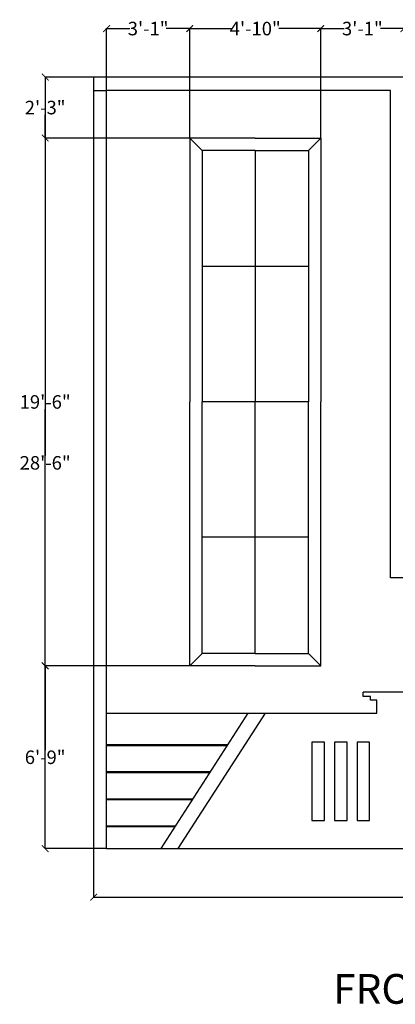
# Model space of a CAD drawing. Units: inches. Extents: x 2278 to 7495, y -71 to 1198.
# Tile 8 of 44: x 4704 to 4871, y -71 to 366. Entities that reach past the tile are written whole.
import ezdxf

# ---------------------------------------------------------------- set-up
doc = ezdxf.new("R2010")
doc.units = ezdxf.units.IN
doc.header["$MEASUREMENT"] = 0
for name, color, linetype, lineweight in [('A-ANNO-DIMS', 2, 'Continuous', 18), ('A-ANNO-TEXT', 7, 'Continuous', 25), ('A-ELEV', 7, 'Continuous', 25)]:
    doc.layers.add(name, color=color, linetype=linetype, lineweight=lineweight)
doc.styles.get("Standard").update_dxf_attribs({"font": 'arial.ttf'})
doc.dimstyles.get("Standard").update_dxf_attribs({"dimtxt": 6, "dimasz": 3, "dimexe": 0.18, "dimexo": 0.0625, "dimgap": 0.09, "dimtad": 0, "dimtih": 1, "dimtoh": 1, "dimdec": 0, "dimzin": 0, "dimdsep": 46, "dimlunit": 3, "dimtxsty": 'Standard', "dimblk": 'ARCHTICK', "dimcen": 0.09, "dimadec": 0, "dimazin": 0, "dimtfac": 1, "dimtdec": 0, "dimtofl": 0, "dimtmove": 0, "dimatfit": 3, "dimfxl": 1, "dimtolj": 1, "dimtzin": 0, "dimarcsym": 0})

# ---------------------------------------------------------------- blocks, each defined once
blk = doc.blocks.new('_ArchTick')
at = {"color": 0, "linetype": 'ByBlock', "const_width": 0.15}
blk.add_lwpolyline([(-0.5, -0.5), (0.5, 0.5)], dxfattribs=at)
blk = doc.blocks.new('*D123')
at = {"layer": 'A-ANNO-DIMS', "color": 0, "lineweight": -2, "transparency": 16777216}
for p, q in [((4736.95, 340.16), (4736.95, -23.43)), ((5145.68, -1.81), (5145.68, -23.43)), ((4736.95, -23.25), (4923.93, -23.25)), ((5145.68, -23.25), (4958.7, -23.25))]:
    blk.add_line(p, q, dxfattribs=at)
at = {"layer": 'Defpoints', "color": 0, "transparency": 16777216}
for p in [(4736.95, 340.22), (5145.68, -1.75), (5145.68, -23.25)]:
    blk.add_point(p, dxfattribs=at)
at = {"layer": 'A-ANNO-DIMS', "color": 0, "lineweight": -2, "transparency": 16777216, "xscale": 3, "yscale": 3, "zscale": 3, "rotation": 180}
blk.add_blockref('_ArchTick', (4736.95, -23.25), dxfattribs=at)
at = {"layer": 'A-ANNO-DIMS', "color": 0, "lineweight": -2, "transparency": 16777216, "xscale": 3, "yscale": 3, "zscale": 3}
blk.add_blockref('_ArchTick', (5145.68, -23.25), dxfattribs=at)
at = {"layer": 'A-ANNO-DIMS', "color": 0, "transparency": 16777216, "insert": (4941.31, -23.25), "char_height": 6, "attachment_point": 5}
blk.add_mtext('\\A1;34\'-0 1/2"', dxfattribs=at)
blk = doc.blocks.new('*D124')
at = {"layer": 'A-ANNO-DIMS', "color": 0, "lineweight": -2, "transparency": 16777216}
for p, q in [((4742.68, 334.28), (4742.68, 361.9)), ((4742.68, 361.72), (4753.08, 361.72)), ((4779.62, 361.72), (4769.21, 361.72)), ((4779.62, 313.27), (4779.62, 361.9))]:
    blk.add_line(p, q, dxfattribs=at)
at = {"layer": 'Defpoints', "color": 0, "transparency": 16777216}
for p in [(4779.62, 361.72), (4742.68, 334.22), (4779.62, 313.21)]:
    blk.add_point(p, dxfattribs=at)
at = {"layer": 'A-ANNO-DIMS', "color": 0, "lineweight": -2, "transparency": 16777216, "xscale": 3, "yscale": 3, "zscale": 3, "rotation": 180}
blk.add_blockref('_ArchTick', (4742.68, 361.72), dxfattribs=at)
at = {"layer": 'A-ANNO-DIMS', "color": 0, "lineweight": -2, "transparency": 16777216, "xscale": 3, "yscale": 3, "zscale": 3}
blk.add_blockref('_ArchTick', (4779.62, 361.72), dxfattribs=at)
at = {"layer": 'A-ANNO-DIMS', "color": 0, "transparency": 16777216, "insert": (4761.15, 361.72), "char_height": 6, "attachment_point": 5}
blk.add_mtext('\\A1;3\'-1"', dxfattribs=at)
blk = doc.blocks.new('*D125')
at = {"layer": 'A-ANNO-DIMS', "color": 0, "lineweight": -2, "transparency": 16777216}
for p, q in [((4779.62, 313.27), (4779.62, 361.9)), ((4779.62, 361.72), (4798.16, 361.72)), ((4837.74, 361.72), (4819.19, 361.72)), ((4837.74, 313.27), (4837.74, 361.9))]:
    blk.add_line(p, q, dxfattribs=at)
at = {"layer": 'Defpoints', "color": 0, "transparency": 16777216}
for p in [(4837.74, 361.72), (4779.62, 313.21), (4837.74, 313.21)]:
    blk.add_point(p, dxfattribs=at)
at = {"layer": 'A-ANNO-DIMS', "color": 0, "lineweight": -2, "transparency": 16777216, "xscale": 3, "yscale": 3, "zscale": 3, "rotation": 180}
blk.add_blockref('_ArchTick', (4779.62, 361.72), dxfattribs=at)
at = {"layer": 'A-ANNO-DIMS', "color": 0, "lineweight": -2, "transparency": 16777216, "xscale": 3, "yscale": 3, "zscale": 3}
blk.add_blockref('_ArchTick', (4837.74, 361.72), dxfattribs=at)
at = {"layer": 'A-ANNO-DIMS', "color": 0, "transparency": 16777216, "insert": (4808.68, 361.72), "char_height": 6, "attachment_point": 5}
blk.add_mtext('\\A1;4\'-10"', dxfattribs=at)
blk = doc.blocks.new('*D126')
at = {"layer": 'A-ANNO-DIMS', "color": 0, "lineweight": -2, "transparency": 16777216}
for p, q in [((4837.74, 313.27), (4837.74, 361.9)), ((4837.74, 361.72), (4848.14, 361.72)), ((4874.68, 361.72), (4864.27, 361.72)), ((4874.68, 99.32), (4874.68, 361.9))]:
    blk.add_line(p, q, dxfattribs=at)
at = {"layer": 'Defpoints', "color": 0, "transparency": 16777216}
for p in [(4874.68, 361.72), (4837.74, 313.21), (4874.68, 99.25)]:
    blk.add_point(p, dxfattribs=at)
at = {"layer": 'A-ANNO-DIMS', "color": 0, "lineweight": -2, "transparency": 16777216, "xscale": 3, "yscale": 3, "zscale": 3, "rotation": 180}
blk.add_blockref('_ArchTick', (4837.74, 361.72), dxfattribs=at)
at = {"layer": 'A-ANNO-DIMS', "color": 0, "lineweight": -2, "transparency": 16777216, "xscale": 3, "yscale": 3, "zscale": 3}
blk.add_blockref('_ArchTick', (4874.68, 361.72), dxfattribs=at)
at = {"layer": 'A-ANNO-DIMS', "color": 0, "transparency": 16777216, "insert": (4856.21, 361.72), "char_height": 6, "attachment_point": 5}
blk.add_mtext('\\A1;3\'-1"', dxfattribs=at)
blk = doc.blocks.new('*D132')
at = {"layer": 'A-ANNO-DIMS', "color": 0, "lineweight": -2, "transparency": 16777216}
for p, q in [((4779.55, 79.26), (4715.27, 79.26)), ((4715.45, 79.26), (4715.45, 41.91)), ((4715.45, -1.75), (4715.45, 35.61)), ((4742.61, -1.75), (4715.27, -1.75))]:
    blk.add_line(p, q, dxfattribs=at)
at = {"layer": 'Defpoints', "color": 0, "transparency": 16777216}
for p in [(4715.45, 79.26), (4779.62, 79.26), (4742.68, -1.75)]:
    blk.add_point(p, dxfattribs=at)
at = {"layer": 'A-ANNO-DIMS', "color": 0, "lineweight": -2, "transparency": 16777216, "xscale": 3, "yscale": 3, "zscale": 3}
for p, rotation in [((4715.45, 79.26), 90), ((4715.45, -1.75), 270)]:
    blk.add_blockref('_ArchTick', p, dxfattribs=dict(at, rotation=rotation))
at = {"layer": 'A-ANNO-DIMS', "color": 0, "transparency": 16777216, "insert": (4715.45, 38.76), "char_height": 6, "attachment_point": 5}
blk.add_mtext('\\A1;6\'-9"', dxfattribs=at)
blk = doc.blocks.new('*D133')
at = {"layer": 'A-ANNO-DIMS', "color": 0, "lineweight": -2, "transparency": 16777216}
for p, q in [((4779.55, 313.21), (4715.27, 313.21)), ((4715.45, 313.21), (4715.45, 199.39)), ((4715.45, 79.26), (4715.45, 193.08)), ((4779.55, 79.26), (4715.27, 79.26))]:
    blk.add_line(p, q, dxfattribs=at)
at = {"layer": 'Defpoints', "color": 0, "transparency": 16777216}
for p in [(4715.45, 313.21), (4779.62, 313.21), (4779.62, 79.26)]:
    blk.add_point(p, dxfattribs=at)
at = {"layer": 'A-ANNO-DIMS', "color": 0, "lineweight": -2, "transparency": 16777216, "xscale": 3, "yscale": 3, "zscale": 3}
for p, rotation in [((4715.45, 313.21), 90), ((4715.45, 79.26), 270)]:
    blk.add_blockref('_ArchTick', p, dxfattribs=dict(at, rotation=rotation))
at = {"layer": 'A-ANNO-DIMS', "color": 0, "transparency": 16777216, "insert": (4715.45, 196.24), "char_height": 6, "attachment_point": 5}
blk.add_mtext('\\A1;19\'-6"', dxfattribs=at)
blk = doc.blocks.new('*D134')
at = {"layer": 'A-ANNO-DIMS', "color": 0, "lineweight": -2, "transparency": 16777216}
for p, q in [((4736.89, 340.22), (4715.27, 340.22)), ((4715.45, 340.22), (4715.45, 329.87)), ((4715.45, 313.21), (4715.45, 323.56)), ((4779.55, 313.21), (4715.27, 313.21))]:
    blk.add_line(p, q, dxfattribs=at)
at = {"layer": 'Defpoints', "color": 0, "transparency": 16777216}
for p in [(4715.45, 340.22), (4736.95, 340.22), (4779.62, 313.21)]:
    blk.add_point(p, dxfattribs=at)
at = {"layer": 'A-ANNO-DIMS', "color": 0, "lineweight": -2, "transparency": 16777216, "xscale": 3, "yscale": 3, "zscale": 3}
for p, rotation in [((4715.45, 340.22), 90), ((4715.45, 313.21), 270)]:
    blk.add_blockref('_ArchTick', p, dxfattribs=dict(at, rotation=rotation))
at = {"layer": 'A-ANNO-DIMS', "color": 0, "transparency": 16777216, "insert": (4715.45, 326.71), "char_height": 6, "attachment_point": 5}
blk.add_mtext('\\A1;2\'-3"', dxfattribs=at)
blk = doc.blocks.new('*D135')
at = {"layer": 'A-ANNO-DIMS', "color": 0, "lineweight": -2, "transparency": 16777216}
for p, q in [((4736.89, 340.22), (4715.27, 340.22)), ((4715.45, 340.22), (4715.45, 172.39)), ((4715.45, -1.75), (4715.45, 166.08)), ((4742.61, -1.75), (4715.27, -1.75))]:
    blk.add_line(p, q, dxfattribs=at)
at = {"layer": 'Defpoints', "color": 0, "transparency": 16777216}
for p in [(4715.45, 340.22), (4736.95, 340.22), (4742.68, -1.75)]:
    blk.add_point(p, dxfattribs=at)
at = {"layer": 'A-ANNO-DIMS', "color": 0, "lineweight": -2, "transparency": 16777216, "xscale": 3, "yscale": 3, "zscale": 3}
for p, rotation in [((4715.45, 340.22), 90), ((4715.45, -1.75), 270)]:
    blk.add_blockref('_ArchTick', p, dxfattribs=dict(at, rotation=rotation))
at = {"layer": 'A-ANNO-DIMS', "color": 0, "transparency": 16777216, "insert": (4715.45, 169.24), "char_height": 6, "attachment_point": 5}
blk.add_mtext('\\A1;28\'-6"', dxfattribs=at)

msp = doc.modelspace()

# ---------------------------------------------------------------- linework, layer by layer
at = {"layer": 'A-ELEV'}
for p, q in [((4742.68, 340.22), (4736.95, 340.22)), ((4736.95, 340.22), (4736.95, 334.22)), ((4881.03, 340.22), (4742.68, 340.22)), ((4736.95, 334.22), (4742.68, 334.22)), ((4868.68, 334.25), (4742.68, 334.22)), ((4742.68, -1.75), (4742.68, 334.22)), ((4868.68, 118.25), (4868.68, 334.25)), ((4808.68, 313.21), (4779.62, 313.21)), ((4779.62, 313.21), (4779.62, 196.24)), ((4779.62, 313.21), (4785.11, 307.71)), ((4808.68, 313.21), (4837.74, 313.21)), ((4837.74, 313.21), (4832.24, 307.71)), ((4837.74, 313.21), (4837.74, 196.24)), ((4808.68, 307.71), (4785.11, 307.71)), ((4785.11, 307.71), (4785.11, 196.24)), ((4808.68, 307.71), (4808.68, 196.24)), ((4808.68, 307.71), (4832.24, 307.71)), ((4808.68, 307.71), (4808.68, 196.24)), ((4832.24, 307.71), (4832.24, 196.24)), ((4832.24, 256.24), (4785.11, 256.24)), ((4779.62, 79.26), (4779.62, 196.24)), ((4832.24, 196.24), (4785.11, 196.24)), ((4832.24, 196.24), (4785.11, 196.24)), ((4785.11, 84.76), (4785.11, 196.24)), ((4808.68, 84.76), (4808.68, 196.24)), ((4808.68, 84.76), (4808.68, 196.24)), ((4832.24, 84.76), (4832.24, 196.24)), ((4837.74, 79.26), (4837.74, 196.24)), ((4832.24, 136.24), (4785.11, 136.24)), ((4874.68, 118.25), (4868.68, 118.25)), ((4785.11, 84.76), (4779.62, 79.26)), ((4808.68, 84.76), (4785.11, 84.76)), ((4808.68, 84.76), (4832.24, 84.76)), ((4832.24, 84.76), (4837.74, 79.26)), ((4808.68, 79.26), (4779.62, 79.26)), ((4808.68, 79.26), (4837.74, 79.26)), ((4856.59, 65.61), (4856.59, 67.61)), ((4880.77, 67.61), (4856.59, 67.61)), ((4859.85, 65.61), (4856.59, 65.61)), ((4859.85, 64.1), (4859.85, 65.61)), ((4862.68, 64.1), (4859.85, 64.1)), ((4862.68, 58.25), (4862.68, 64.1)), ((4742.68, 58.25), (4862.68, 58.25)), ((4805.45, 58.25), (4766.71, -1.75)), ((4813.02, 58.25), (4774.28, -1.75)), ((4796.27, 44.24), (4742.68, 44.24)), ((4796.14, 43.84), (4742.68, 43.84)), ((4796.27, 44.24), (4796.27, 44.04)), ((4788.65, 32.24), (4742.68, 32.24)), ((4788.39, 31.84), (4742.68, 31.84)), ((4780.9, 20.24), (4742.68, 20.24)), ((4780.65, 19.84), (4742.68, 19.84)), ((4773.16, 8.24), (4742.68, 8.24)), ((4772.9, 7.84), (4742.68, 7.84)), ((4742.68, -1.75), (5145.68, -1.75))]:
    msp.add_line(p, q, dxfattribs=at)
for points in [[(4839.43, 45.42), (4833.85, 45.42), (4833.85, 10.78), (4839.43, 10.78)], [(4849.43, 45.42), (4843.85, 45.42), (4843.85, 10.78), (4849.43, 10.78)], [(4859.43, 45.42), (4853.85, 45.42), (4853.85, 10.78), (4859.43, 10.78)]]:
    msp.add_lwpolyline(points, close=True, dxfattribs=at)

# ---------------------------------------------------------------- texts
at = {"layer": 'A-ANNO-TEXT'}
msp.add_text('FRONT ELEVATION', height=13.1927, dxfattribs=at).set_placement((4843.31, -70.51))

# ---------------------------------------------------------------- dimensions: what is measured, and where the dimension line sits
at = {"layer": 'A-ANNO-DIMS'}
for base, p1, p2, picture, middle in [((4779.62, 361.72), (4742.68, 334.22), (4779.62, 313.21), '*D124', (4761.15, 361.72)), ((4837.74, 361.72), (4779.62, 313.21), (4837.74, 313.21), '*D125', (4808.68, 361.72)), ((4874.68, 361.72), (4837.74, 313.21), (4874.68, 99.25), '*D126', (4856.21, 361.72)), ((5145.68, -23.25), (4736.95, 340.22), (5145.68, -1.75), '*D123', (4941.31, -23.25))]:
    dim = msp.add_linear_dim(base=base, p1=p1, p2=p2, dimstyle='Standard', override={"dimdec": 1, "dimlfac": 1, "dimrnd": 0, "dimzin": 1, "dimdsep": 46, "dimlunit": 4, "dimfrac": 2}, dxfattribs=at)
    dim.commit()
    dim.dimension.update_dxf_attribs({"geometry": picture, "text_midpoint": middle})
for base, p1, p2, picture, middle in [((4715.45, 340.22), (4742.68, -1.75), (4736.95, 340.22), '*D135', (4715.45, 169.24)), ((4715.45, 340.22), (4779.62, 313.21), (4736.95, 340.22), '*D134', (4715.45, 326.71)), ((4715.45, 313.2079), (4779.6169, 79.2641), (4779.6169, 313.2079), '*D133', (4715.45, 196.236)), ((4715.45, 79.26), (4742.68, -1.75), (4779.62, 79.26), '*D132', (4715.45, 38.76))]:
    dim = msp.add_linear_dim(base=base, p1=p1, p2=p2, angle=90, dimstyle='Standard', override={"dimdec": 1, "dimlfac": 1, "dimrnd": 0, "dimzin": 1, "dimdsep": 46, "dimlunit": 4, "dimfrac": 2}, dxfattribs=at)
    dim.commit()
    dim.dimension.update_dxf_attribs({"geometry": picture, "text_midpoint": middle})

doc.saveas('drawing.dxf')
